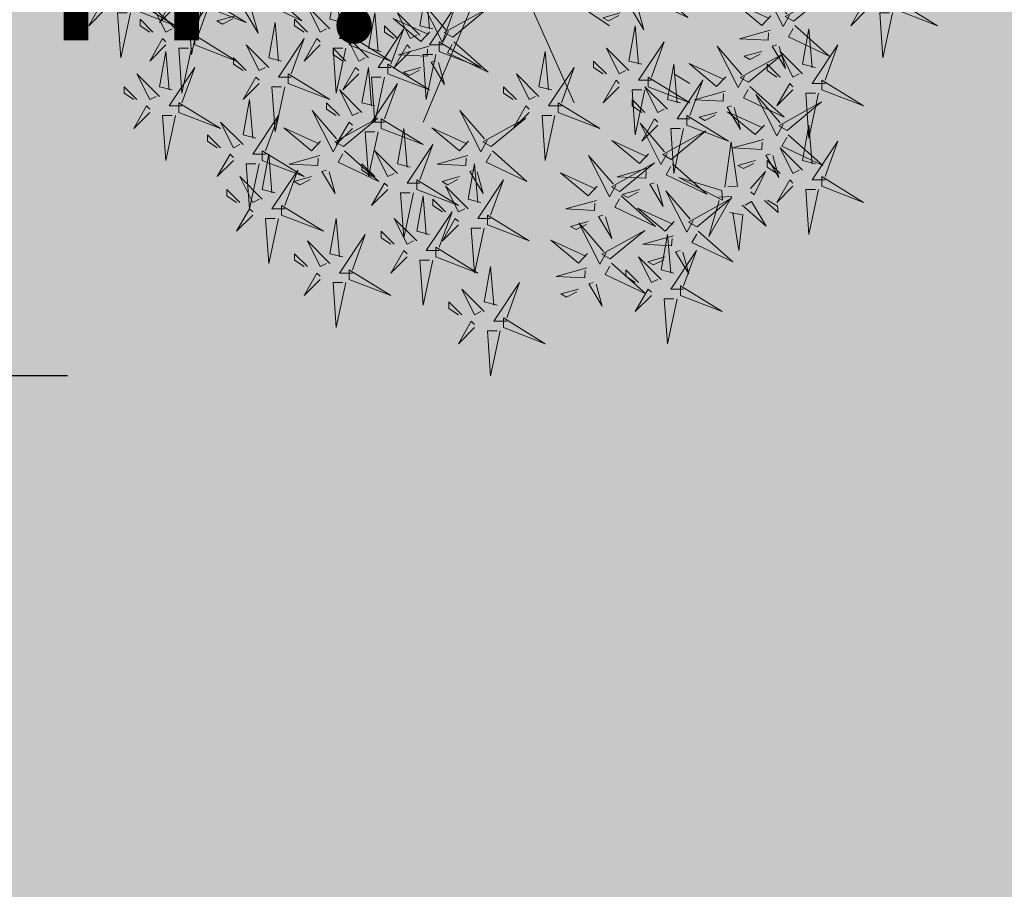
# Model space of a CAD drawing. Units: inches. Extents: x 1704 to 6393, y -157 to 1172.
# Tile 76 of 122: x 2017 to 2048, y 983 to 1009. Entities that reach past the tile are written whole.
import ezdxf

# ---------------------------------------------------------------- set-up
doc = ezdxf.new("R2010")
doc.units = ezdxf.units.IN
doc.header["$MEASUREMENT"] = 0
doc.layers.add('A-ANNO-DIMS', color=7, linetype='Continuous', lineweight=13)
doc.layers.add('L-shrub', color=74, linetype='Continuous', lineweight=18)
doc.layers.add('L-HRDS-PATT', color=9, linetype='Continuous', lineweight=13, true_color=0xc5c1ba)
doc.styles.get("Standard").update_dxf_attribs({"font": 'arial.ttf'})
doc.dimstyles.get("Standard").update_dxf_attribs({"dimtxt": 6, "dimasz": 2, "dimexe": 0.18, "dimexo": 0.0625, "dimgap": 0.09, "dimtad": 0, "dimtih": 1, "dimtoh": 1, "dimdec": 1, "dimzin": 0, "dimdsep": 46, "dimlunit": 3, "dimtxsty": 'Standard', "dimblk": 'ARCHTICK', "dimcen": 0.09, "dimadec": 0, "dimazin": 0, "dimtfac": 1, "dimtdec": 1, "dimtofl": 0, "dimtmove": 0, "dimatfit": 3, "dimfxl": 1, "dimtolj": 1, "dimtzin": 0, "dimarcsym": 0})

# ---------------------------------------------------------------- blocks, each defined once
blk = doc.blocks.new('autumn shrub')
at = {"layer": 'L-shrub'}
for p, q in [((11.54, 1.92), (51.94, 98)), ((1.92, -3.84), (-38.48, 86.47)), ((-98.12, 69.17), (-107.74, 74.94)), ((0, 0), (-59.64, 40.35)), ((71.18, 17.29), (98.12, 26.9)), ((9.62, -3.84), (71.18, 17.29)), ((11.54, -5.76), (55.79, 0)), ((-5.77, -9.61), (-38.48, -19.21)), ((1.92, -13.45), (-15.39, -86.47)), ((17.31, -26.9), (25.01, -40.35)), ((-76.95, -34.59), (-126.97, -48.04)), ((-67.33, -57.64), (-80.8, -63.41)), ((46.17, -69.17), (63.49, -101.84)), ((-17.31, -122.97), (-23.09, -155.64))]:
    blk.add_line(p, q, dxfattribs=at)
for points in [[(5.77, 222.89), (11.54, 249.79), (13.47, 222.89), (7.7, 222.89)], [(-100.04, 203.68), (-94.27, 230.58), (-92.34, 203.68), (-98.12, 203.68)], [(3.85, 220.97), (-21.16, 230.58), (3.85, 215.21), (3.85, 220.97)], [(21.16, 220.97), (30.78, 230.58), (23.09, 217.13), (21.16, 219.05)], [(98.12, 194.07), (103.89, 220.97), (105.81, 194.07), (100.04, 194.07)], [(1.92, 217.13), (9.62, 217.13), (-5.77, 194.07), (1.92, 215.21)], [(15.39, 211.36), (28.86, 197.91), (21.16, 213.28), (17.31, 211.36)], [(28.86, 213.28), (36.55, 205.6), (36.55, 209.44), (30.78, 213.28)], [(-101.96, 201.75), (-126.97, 211.36), (-101.96, 195.99), (-101.96, 201.75)], [(-84.65, 201.75), (-75.03, 211.36), (-82.73, 197.91), (-84.65, 199.83)], [(-51.51, 194.97), (-55.15, 208.07), (-47.22, 194.76), (-49.84, 194.03)], [(7.7, 207.52), (15.39, 205.6), (11.54, 184.46), (9.62, 207.52)], [(46.17, 180.62), (51.94, 207.52), (53.87, 180.62), (48.1, 180.62)], [(-60.75, 182.51), (-81.34, 200.76), (-56.96, 189.22), (-59.8, 184.19)], [(-41.04, 197.9), (-30.56, 200.83), (-33.91, 202.71), (-40.09, 199.58)], [(96.19, 192.15), (71.18, 201.75), (96.19, 186.38), (96.19, 192.15)], [(113.51, 192.15), (123.13, 201.75), (115.43, 188.3), (113.51, 190.23)], [(-103.89, 197.91), (-96.19, 197.91), (-111.58, 174.85), (-103.89, 195.99)], [(-103.45, 175.76), (-107.1, 188.86), (-99.16, 175.55), (-101.78, 174.81)], [(-90.42, 192.15), (-76.95, 178.7), (-84.65, 194.07), (-88.5, 192.15)], [(-76.95, 194.07), (-69.26, 186.38), (-69.26, 190.23), (-75.03, 194.07)], [(-45.98, 185.23), (-27.65, 190.35), (-44.82, 191.2), (-45.03, 186.9)], [(-98.12, 188.3), (-90.42, 186.38), (-94.27, 165.25), (-96.19, 188.3)], [(-92.98, 178.69), (-82.5, 181.61), (-85.85, 183.5), (-92.03, 180.36)], [(-57.62, 176.33), (-53.83, 183.03), (-41.31, 158.3), (-55.94, 175.38)], [(15.39, 161.4), (21.16, 188.3), (23.09, 161.4), (17.31, 161.4)], [(44.25, 178.7), (19.24, 188.3), (44.25, 172.93), (44.25, 178.7)], [(61.56, 178.7), (71.18, 188.3), (63.49, 174.85), (61.56, 176.78)], [(94.27, 188.3), (101.96, 188.3), (86.57, 165.25), (94.27, 186.38)], [(107.74, 182.54), (121.2, 169.09), (113.51, 184.46), (109.66, 182.54)], [(121.2, 184.46), (128.9, 176.78), (128.9, 180.62), (123.13, 184.46)], [(-112.69, 163.3), (-133.28, 181.54), (-108.91, 170), (-111.74, 164.97)], [(-60.02, 179.89), (-80.67, 162.83), (-55, 177.06), (-60.02, 179.89)], [(-46.41, 176.64), (-40.96, 182.39), (-24.44, 168.66), (-45.47, 178.31)], [(100.04, 178.7), (107.74, 176.78), (103.89, 155.64), (101.96, 178.7)], [(138.52, 155.64), (144.29, 182.54), (146.21, 155.64), (140.44, 155.64)], [(-131.51, 152.18), (-139.33, 153.55), (-136.98, 174.91), (-133.43, 152.04)], [(-97.92, 166.01), (-79.59, 171.13), (-96.76, 171.98), (-96.98, 167.69)], [(42.32, 174.85), (50.02, 174.85), (34.63, 151.8), (42.32, 172.93)], [(55.79, 169.09), (69.26, 155.64), (61.56, 171.01), (57.72, 169.09)], [(69.26, 171.01), (76.95, 163.33), (76.95, 167.17), (71.18, 171.01)], [(-184.69, 138.35), (-178.92, 165.25), (-176.99, 138.35), (-182.77, 138.35)], [(-125.08, 143), (-132.76, 142.46), (-119.03, 166.55), (-125.21, 144.92)], [(-57.28, 154.62), (-60.92, 167.72), (-52.99, 154.41), (-55.61, 153.68)], [(13.47, 159.48), (-11.54, 169.09), (13.47, 153.72), (13.47, 159.48)], [(30.78, 159.48), (40.4, 169.09), (32.71, 155.64), (30.78, 157.56)], [(48.1, 165.25), (55.79, 163.33), (51.94, 142.19), (50.02, 165.25)], [(57.72, 140.27), (63.49, 167.17), (65.41, 140.27), (59.64, 140.27)], [(-138.92, 147.8), (-153.3, 160.27), (-144.54, 145.48), (-140.84, 147.67)], [(-111.96, 160.68), (-132.62, 143.61), (-106.94, 157.85), (-111.96, 160.68)], [(-109.56, 157.11), (-105.78, 163.82), (-93.26, 139.08), (-107.89, 156.17)], [(-98.36, 157.42), (-92.9, 163.18), (-76.38, 149.44), (-97.41, 159.1)], [(-66.52, 142.16), (-87.11, 160.4), (-62.74, 148.86), (-65.57, 143.84)], [(-46.81, 157.55), (-36.33, 160.48), (-39.68, 162.36), (-45.86, 159.22)], [(136.59, 153.72), (111.58, 163.33), (136.59, 147.95), (136.59, 153.72)], [(153.91, 153.72), (163.53, 163.33), (155.83, 149.87), (153.91, 151.8)], [(11.54, 155.64), (19.24, 155.64), (3.85, 132.58), (11.54, 153.72)], [(-152.22, 144.94), (-160.44, 152.06), (-160.16, 148.23), (-154.14, 144.8)], [(-88.06, 135.41), (-91.71, 148.51), (-83.77, 135.2), (-86.39, 134.46)], [(-51.75, 144.88), (-33.42, 150), (-50.59, 150.85), (-50.8, 146.55)], [(25.01, 149.87), (38.48, 136.42), (30.78, 151.8), (26.93, 149.87)], [(55.79, 138.35), (30.78, 147.95), (55.79, 132.58), (55.79, 138.35)], [(38.48, 151.8), (46.17, 144.11), (46.17, 147.95), (40.4, 151.8)], [(73.11, 138.35), (82.73, 147.95), (75.03, 134.5), (73.11, 136.42)], [(134.67, 149.87), (142.36, 149.87), (126.97, 126.82), (134.67, 147.95)], [(150.06, 122.97), (155.83, 149.87), (157.76, 122.97), (151.98, 122.97)], [(-186.61, 136.42), (-211.62, 146.03), (-186.61, 130.66), (-186.61, 136.42)], [(-169.3, 136.42), (-159.68, 146.03), (-167.38, 132.58), (-169.3, 134.5)], [(-144, 137.81), (-152.92, 127.55), (-146.19, 141.51), (-144.13, 139.73)], [(-126.73, 139.03), (-101.1, 131.22), (-127.13, 144.78), (-126.73, 139.03)], [(-77.59, 138.33), (-67.11, 141.26), (-70.46, 143.15), (-76.64, 140.01)], [(-63.39, 135.98), (-59.61, 142.68), (-47.08, 117.95), (-61.71, 135.03)], [(-52.18, 136.28), (-46.73, 142.04), (-30.21, 128.31), (-51.24, 137.96)], [(17.31, 146.03), (25.01, 144.11), (21.16, 122.97), (19.24, 146.03)], [(148.14, 144.11), (161.6, 130.66), (153.91, 146.03), (150.06, 144.11)], [(161.6, 146.03), (169.3, 138.35), (169.3, 142.19), (163.53, 146.03)], [(-128.51, 136.98), (-132.37, 109.74), (-136.19, 136.44), (-130.43, 136.85)], [(-97.3, 122.95), (-117.89, 141.19), (-93.52, 129.65), (-96.35, 124.62)], [(-65.79, 139.54), (-86.44, 122.48), (-60.77, 136.71), (-65.79, 139.54)], [(19.67, 127.72), (16.03, 140.82), (23.96, 127.51), (21.35, 126.78)], [(108.17, 127.72), (104.53, 140.82), (112.46, 127.51), (109.84, 126.78)], [(140.44, 140.27), (148.14, 138.35), (144.29, 117.21), (142.36, 140.27)], [(-188.54, 132.58), (-180.84, 132.58), (-196.23, 109.52), (-188.54, 130.66)], [(-157.32, 118.11), (-160.96, 131.21), (-153.03, 117.9), (-155.65, 117.17)], [(-82.53, 125.66), (-64.2, 130.78), (-81.37, 131.63), (-81.59, 127.34)], [(10.44, 115.26), (-10.16, 133.5), (14.22, 121.96), (11.38, 116.94)], [(30.15, 130.65), (40.62, 133.58), (37.28, 135.46), (31.09, 132.32)], [(53.87, 134.5), (61.56, 134.5), (46.17, 111.45), (53.87, 132.58)], [(67.33, 128.74), (80.8, 115.29), (73.11, 130.66), (69.26, 128.74)], [(98.93, 115.26), (78.34, 133.5), (102.71, 121.96), (99.88, 116.94)], [(78.88, 103.76), (84.65, 130.66), (86.57, 103.76), (80.8, 103.76)], [(80.8, 130.66), (88.5, 122.97), (88.5, 126.82), (82.73, 130.66)], [(118.64, 130.65), (129.12, 133.58), (125.77, 135.46), (119.59, 132.32)], [(148.14, 121.05), (123.13, 130.66), (148.14, 115.29), (148.14, 121.05)], [(165.45, 121.05), (175.07, 130.66), (167.38, 117.21), (165.45, 119.13)], [(-166.56, 105.65), (-187.15, 123.9), (-162.78, 112.36), (-165.61, 107.33)], [(-175.07, 126.82), (-161.6, 113.37), (-169.3, 128.74), (-173.15, 126.82)], [(-161.6, 128.74), (-153.91, 121.05), (-153.91, 124.9), (-159.68, 128.74)], [(-146.85, 121.04), (-136.37, 123.97), (-139.72, 125.86), (-145.9, 122.72)], [(-103.89, 101.84), (-98.12, 128.74), (-96.19, 101.84), (-101.96, 101.84)], [(25.2, 117.98), (43.54, 123.1), (26.37, 123.95), (26.15, 119.65)], [(59.64, 124.9), (67.33, 122.97), (63.49, 101.84), (61.56, 124.9)], [(113.7, 117.98), (132.03, 123.1), (114.86, 123.95), (114.65, 119.65)], [(-182.77, 122.97), (-175.07, 121.05), (-178.92, 99.92), (-180.84, 122.97)], [(-96.57, 120.33), (-117.23, 103.26), (-91.55, 117.49), (-96.57, 120.33)], [(-94.17, 116.76), (-90.39, 123.47), (-77.87, 98.73), (-92.49, 115.82)], [(-82.96, 117.07), (-77.51, 122.83), (-60.99, 109.09), (-82.02, 118.75)], [(-26.93, 94.15), (-21.16, 121.05), (-19.24, 94.15), (-25.01, 94.15)], [(200.08, 94.15), (205.85, 121.05), (207.78, 94.15), (202, 94.15)], [(-151.79, 108.37), (-133.46, 113.49), (-150.63, 114.34), (-150.84, 110.04)], [(11.17, 112.64), (-9.49, 95.58), (16.19, 109.81), (11.17, 112.64)], [(13.57, 109.08), (17.35, 115.78), (29.87, 91.05), (15.24, 108.13)], [(24.77, 109.38), (30.23, 115.14), (46.74, 101.41), (25.72, 111.06)], [(99.66, 112.64), (79.01, 95.58), (104.68, 109.81), (99.66, 112.64)], [(102.06, 109.08), (105.85, 115.78), (118.37, 91.05), (103.74, 108.13)], [(113.27, 109.38), (118.72, 115.14), (135.24, 101.41), (114.21, 111.06)], [(146.21, 117.21), (153.91, 117.21), (138.52, 94.15), (146.21, 115.29)], [(159.68, 111.45), (173.15, 98), (165.45, 113.37), (161.6, 111.45)], [(173.15, 113.37), (180.84, 105.68), (180.84, 109.52), (175.07, 113.37)], [(-184.69, 80.7), (-178.92, 107.6), (-176.99, 80.7), (-182.77, 80.7)], [(-163.43, 99.47), (-159.65, 106.17), (-147.12, 81.44), (-161.75, 98.53)], [(-105.81, 99.92), (-130.82, 109.52), (-105.81, 94.15), (-105.81, 99.92)], [(-88.5, 99.92), (-78.88, 109.52), (-86.57, 96.07), (-88.5, 98)], [(76.95, 101.84), (51.94, 111.45), (76.95, 96.07), (76.95, 101.84)], [(94.27, 101.84), (103.89, 111.45), (96.19, 98), (94.27, 99.92)], [(151.98, 107.6), (159.68, 105.68), (155.83, 84.54), (153.91, 107.6)], [(-165.83, 103.03), (-186.48, 85.97), (-160.81, 100.2), (-165.83, 103.03)], [(-152.22, 99.78), (-146.77, 105.54), (-130.25, 91.8), (-151.28, 101.45)], [(-134.24, 89.29), (-137.88, 102.39), (-129.94, 89.08), (-132.56, 88.35)], [(-80.8, 78.78), (-75.03, 105.68), (-73.11, 78.78), (-78.88, 78.78)], [(-28.86, 92.23), (-53.87, 101.84), (-28.86, 86.47), (-28.86, 92.23)], [(-11.54, 92.23), (-1.92, 101.84), (-9.62, 88.39), (-11.54, 90.31)], [(134.67, 76.86), (140.44, 103.76), (142.36, 76.86), (136.59, 76.86)], [(198.16, 92.23), (173.15, 101.84), (198.16, 86.47), (198.16, 92.23)], [(215.47, 92.23), (225.09, 101.84), (217.4, 88.39), (215.47, 90.31)], [(-143.47, 76.83), (-164.07, 95.07), (-139.69, 83.53), (-142.53, 78.51)], [(-123.76, 92.22), (-113.29, 95.15), (-116.63, 97.03), (-122.82, 93.89)], [(-107.74, 96.07), (-100.04, 96.07), (-115.43, 73.02), (-107.74, 94.15)], [(75.03, 98), (82.73, 98), (67.33, 74.94), (75.03, 96.07)], [(75.03, 71.09), (80.8, 98), (82.73, 71.09), (76.95, 71.09)], [(-186.61, 78.78), (-211.62, 88.39), (-186.61, 73.02), (-186.61, 78.78)], [(-169.3, 78.78), (-159.68, 88.39), (-167.38, 74.94), (-169.3, 76.86)], [(-94.27, 90.31), (-80.8, 76.86), (-88.5, 92.23), (-92.34, 90.31)], [(-80.8, 92.23), (-73.11, 84.54), (-73.11, 88.39), (-78.88, 92.23)], [(-30.78, 88.39), (-23.09, 88.39), (-38.48, 65.33), (-30.78, 86.47)], [(80.8, 88.39), (88.5, 86.47), (84.65, 65.33), (82.73, 88.39)], [(88.5, 92.23), (101.96, 78.78), (94.27, 94.15), (90.42, 92.23)], [(101.96, 94.15), (109.66, 86.47), (109.66, 90.31), (103.89, 94.15)], [(196.23, 88.39), (203.93, 88.39), (188.54, 65.33), (196.23, 86.47)], [(-128.7, 79.55), (-110.37, 84.67), (-127.54, 85.52), (-127.76, 81.22)], [(-82.73, 76.86), (-107.74, 86.47), (-82.73, 71.09), (-82.73, 76.86)], [(-101.96, 86.47), (-94.27, 84.54), (-98.12, 63.41), (-100.04, 86.47)], [(-65.41, 76.86), (-55.79, 86.47), (-63.49, 73.02), (-65.41, 74.94)], [(-17.31, 82.62), (-3.85, 69.17), (-11.54, 84.54), (-15.39, 82.62)], [(-3.85, 84.54), (3.85, 76.86), (3.85, 80.7), (-1.92, 84.54)], [(44.25, 57.64), (50.02, 84.54), (51.94, 57.64), (46.17, 57.64)], [(132.75, 74.94), (107.74, 84.54), (132.75, 69.17), (132.75, 74.94)], [(150.06, 74.94), (159.68, 84.54), (151.98, 71.09), (150.06, 73.02)], [(209.7, 82.62), (223.17, 69.17), (215.47, 84.54), (211.62, 82.62)], [(223.17, 84.54), (230.86, 76.86), (230.86, 80.7), (225.09, 84.54)], [(-140.34, 70.65), (-136.56, 77.35), (-124.04, 52.62), (-138.67, 69.7)], [(-129.14, 70.95), (-123.68, 76.71), (-107.16, 62.98), (-128.19, 72.63)], [(-25.01, 78.78), (-17.31, 76.86), (-21.16, 55.72), (-23.09, 78.78)], [(73.11, 69.17), (48.1, 78.78), (73.11, 63.41), (73.11, 69.17)], [(90.42, 69.17), (100.04, 78.78), (92.34, 65.33), (90.42, 67.25)], [(98.12, 53.8), (103.89, 80.7), (105.81, 53.8), (100.04, 53.8)], [(190.46, 53.8), (196.23, 80.7), (198.16, 53.8), (192.39, 53.8)], [(202, 78.78), (209.7, 76.86), (205.85, 55.72), (203.93, 78.78)], [(-188.54, 74.94), (-180.84, 74.94), (-196.23, 51.88), (-188.54, 73.02)], [(-175.07, 69.17), (-161.6, 55.72), (-169.3, 71.09), (-173.15, 69.17)], [(-142.74, 74.21), (-163.4, 57.15), (-137.72, 71.38), (-142.74, 74.21)], [(-161.6, 71.09), (-153.91, 63.41), (-153.91, 67.25), (-159.68, 71.09)], [(-84.65, 73.02), (-76.95, 73.02), (-92.34, 49.96), (-84.65, 71.09)], [(42.76, 62.39), (39.12, 75.49), (47.05, 62.18), (44.43, 61.45)], [(130.82, 71.09), (138.52, 71.09), (123.13, 48.04), (130.82, 69.17)], [(-182.77, 65.33), (-175.07, 63.41), (-178.92, 42.27), (-180.84, 65.33)], [(-161.17, 52.78), (-164.81, 65.88), (-156.88, 52.57), (-159.5, 51.84)], [(-71.18, 67.25), (-57.72, 53.8), (-65.41, 69.17), (-69.26, 67.25)], [(-57.72, 69.17), (-50.02, 61.49), (-50.02, 65.33), (-55.79, 69.17)], [(33.52, 49.93), (12.93, 68.17), (37.3, 56.63), (34.47, 51.61)], [(42.32, 55.72), (17.31, 65.33), (42.32, 49.96), (42.32, 55.72)], [(53.23, 65.32), (63.71, 68.25), (60.36, 70.13), (54.18, 66.99)], [(59.64, 55.72), (69.26, 65.33), (61.56, 51.88), (59.64, 53.8)], [(71.18, 65.33), (78.88, 65.33), (63.49, 42.27), (71.18, 63.41)], [(144.29, 65.33), (157.76, 51.88), (150.06, 67.25), (146.21, 65.33)], [(157.76, 67.25), (165.45, 59.57), (165.45, 63.41), (159.68, 67.25)], [(-228.94, 32.67), (-223.17, 59.57), (-221.24, 32.67), (-227.01, 32.67)], [(-150.69, 55.71), (-140.22, 58.64), (-143.57, 60.53), (-149.75, 57.39)], [(-78.88, 63.41), (-71.18, 61.49), (-75.03, 40.35), (-76.95, 63.41)], [(96.19, 51.88), (71.18, 61.49), (96.19, 46.12), (96.19, 51.88)], [(84.65, 59.57), (98.12, 46.12), (90.42, 61.49), (86.57, 59.57)], [(98.12, 61.49), (105.81, 53.8), (105.81, 57.64), (100.04, 61.49)], [(113.51, 51.88), (123.13, 61.49), (115.43, 48.04), (113.51, 49.96)], [(136.59, 61.49), (144.29, 59.57), (140.44, 38.43), (138.52, 61.49)], [(188.54, 51.88), (163.53, 61.49), (188.54, 46.12), (188.54, 51.88)], [(205.85, 51.88), (215.47, 61.49), (207.78, 48.04), (205.85, 49.96)], [(227.01, 32.67), (232.79, 59.57), (234.71, 32.67), (228.94, 32.67)], [(-170.4, 40.32), (-191, 58.57), (-166.62, 47.03), (-169.46, 42)], [(48.29, 52.64), (66.62, 57.77), (49.45, 58.62), (49.24, 54.32)], [(76.95, 55.72), (84.65, 53.8), (80.8, 32.67), (78.88, 55.72)], [(184.69, 30.74), (190.46, 57.64), (192.39, 30.74), (186.61, 30.74)], [(-155.64, 43.04), (-137.31, 48.16), (-154.48, 49.01), (-154.69, 44.71)], [(34.25, 47.31), (13.6, 30.25), (39.27, 44.48), (34.25, 47.31)], [(40.4, 51.88), (48.1, 51.88), (32.71, 28.82), (40.4, 49.96)], [(36.65, 43.75), (40.43, 50.45), (52.96, 25.72), (38.33, 42.8)], [(47.86, 44.05), (53.31, 49.81), (69.83, 36.08), (48.8, 45.73)], [(53.87, 46.12), (67.33, 32.67), (59.64, 48.04), (55.79, 46.12)], [(67.33, 48.04), (75.03, 40.35), (75.03, 44.19), (69.26, 48.04)], [(94.27, 48.04), (101.96, 48.04), (86.57, 24.98), (94.27, 46.12)], [(186.61, 48.04), (194.31, 48.04), (178.92, 24.98), (186.61, 46.12)], [(-76.52, 29.73), (-80.16, 42.83), (-72.23, 29.51), (-74.85, 28.78)], [(46.17, 42.27), (53.87, 40.35), (50.02, 19.21), (48.1, 42.27)], [(107.74, 42.27), (121.2, 28.82), (113.51, 44.19), (109.66, 42.27)], [(121.2, 44.19), (128.9, 36.51), (128.9, 40.35), (123.13, 44.19)], [(154.34, 31.65), (150.7, 44.75), (158.63, 31.44), (156.02, 30.7)], [(200.08, 42.27), (213.55, 28.82), (205.85, 44.19), (202, 42.27)], [(213.55, 44.19), (221.24, 36.51), (221.24, 40.35), (215.47, 44.19)], [(-230.86, 30.74), (-255.87, 40.35), (-230.86, 24.98), (-230.86, 30.74)], [(-213.55, 30.74), (-203.93, 40.35), (-211.62, 26.9), (-213.55, 28.82)], [(-169.68, 37.7), (-190.33, 20.64), (-164.66, 34.87), (-169.68, 37.7)], [(-167.27, 34.14), (-163.49, 40.84), (-150.97, 16.11), (-165.6, 33.2)], [(-156.07, 34.45), (-150.62, 40.21), (-134.1, 26.47), (-155.13, 36.12)], [(-85.76, 17.27), (-106.35, 35.51), (-81.97, 23.97), (-84.81, 18.94)], [(-66.05, 32.65), (-55.57, 35.58), (-58.92, 37.47), (-65.1, 34.33)], [(100.04, 38.43), (107.74, 36.51), (103.89, 15.37), (101.96, 38.43)], [(145.11, 19.19), (124.51, 37.43), (148.89, 25.89), (146.05, 20.86)], [(182.77, 28.82), (157.76, 38.43), (182.77, 23.06), (182.77, 28.82)], [(164.82, 34.57), (175.29, 37.5), (171.94, 39.39), (165.76, 36.25)], [(192.39, 38.43), (200.08, 36.51), (196.23, 15.37), (194.31, 38.43)], [(225.09, 30.74), (200.08, 40.35), (225.09, 24.98), (225.09, 30.74)], [(200.08, 28.82), (209.7, 38.43), (202, 24.98), (200.08, 26.9)], [(242.41, 30.74), (252.02, 40.35), (244.33, 26.9), (242.41, 28.82)], [(-232.79, 26.9), (-225.09, 26.9), (-240.48, 3.84), (-232.79, 24.98)], [(-70.99, 19.98), (-52.66, 25.1), (-69.83, 25.95), (-70.04, 21.66)], [(159.87, 21.9), (178.21, 27.02), (161.04, 27.87), (160.82, 23.58)], [(180.84, 24.98), (188.54, 24.98), (173.15, 1.92), (180.84, 23.06)], [(223.17, 26.9), (230.86, 26.9), (215.47, 3.84), (223.17, 24.98)], [(215.47, -1.92), (221.24, 24.98), (223.17, -1.92), (217.4, -1.92)], [(-219.32, 21.14), (-205.85, 7.69), (-213.55, 23.06), (-217.4, 21.14)], [(-213.55, -3.84), (-207.78, 23.06), (-205.85, -3.84), (-211.62, -3.84)], [(-205.85, 23.06), (-198.16, 15.37), (-198.16, 19.21), (-203.93, 23.06)], [(-161.6, -7.69), (-155.83, 19.21), (-153.91, -7.69), (-159.68, -7.69)], [(-96.19, -5.76), (-90.42, 21.14), (-88.5, -5.76), (-94.27, -5.76)], [(-82.63, 11.08), (-78.84, 17.78), (-66.32, -6.95), (-80.95, 10.14)], [(-57.72, -3.84), (-51.94, 23.06), (-50.02, -3.84), (-55.79, -3.84)], [(148.24, 13), (152.02, 19.71), (164.54, -5.03), (149.91, 12.06)], [(159.44, 13.31), (164.89, 19.07), (181.41, 5.33), (160.39, 14.99)], [(194.31, 19.21), (207.78, 5.76), (200.08, 21.14), (196.23, 19.21)], [(207.78, 21.14), (215.47, 13.45), (215.47, 17.29), (209.7, 21.14)], [(236.63, 21.14), (250.1, 7.69), (242.41, 23.06), (238.56, 21.14)], [(250.1, 23.06), (257.8, 15.37), (257.8, 19.21), (252.02, 23.06)], [(-227.01, 17.29), (-219.32, 15.37), (-223.17, -5.76), (-225.09, 17.29)], [(-85.03, 14.65), (-105.68, -2.42), (-80.01, 11.81), (-85.03, 14.65)], [(-71.42, 11.39), (-65.97, 17.15), (-49.45, 3.41), (-70.48, 13.06)], [(34.63, -9.61), (40.4, 17.29), (42.32, -9.61), (36.55, -9.61)], [(145.83, 16.57), (125.18, -0.5), (150.86, 13.74), (145.83, 16.57)], [(186.61, 15.37), (194.31, 13.45), (190.46, -7.69), (188.54, 15.37)], [(228.94, 17.29), (236.63, 15.37), (232.79, -5.76), (230.86, 17.29)], [(-215.47, -5.76), (-240.48, 3.84), (-215.47, -11.53), (-215.47, -5.76)], [(-198.16, -5.76), (-188.54, 3.84), (-196.23, -9.61), (-198.16, -7.69)], [(-163.53, -9.61), (-188.54, 0), (-163.53, -15.37), (-163.53, -9.61)], [(-146.21, -9.61), (-136.59, 0), (-144.29, -13.45), (-146.21, -11.53)], [(-98.12, -7.69), (-123.13, 1.92), (-98.12, -13.45), (-98.12, -7.69)], [(-59.64, -5.76), (-84.65, 3.84), (-59.64, -11.53), (-59.64, -5.76)], [(-80.8, -7.69), (-71.18, 1.92), (-78.88, -11.53), (-80.8, -9.61)], [(-42.32, -5.76), (-32.71, 3.84), (-40.4, -9.61), (-42.32, -7.69)], [(110.09, -10.62), (106.45, 2.47), (114.39, -10.84), (111.77, -11.57)], [(213.55, -3.84), (188.54, 5.76), (213.55, -9.61), (213.55, -3.84)], [(230.86, -3.84), (240.48, 5.76), (232.79, -7.69), (230.86, -5.76)], [(232.79, -26.9), (238.56, 0), (240.48, -26.9), (234.71, -26.9)], [(32.71, -11.53), (7.7, -1.92), (32.71, -17.29), (32.71, -11.53)], [(50.02, -11.53), (59.64, -1.92), (51.94, -15.37), (50.02, -13.45)], [(100.86, -23.09), (80.26, -4.84), (104.64, -16.38), (101.8, -21.41)], [(120.57, -7.7), (131.04, -4.77), (127.7, -2.88), (121.51, -6.02)], [(-217.4, -9.61), (-209.7, -9.61), (-225.09, -32.67), (-217.4, -11.53)], [(-100.04, -11.53), (-92.34, -11.53), (-107.74, -34.59), (-100.04, -13.45)], [(-61.56, -9.61), (-53.87, -9.61), (-69.26, -32.67), (-61.56, -11.53)], [(211.62, -7.69), (219.32, -7.69), (203.93, -30.74), (211.62, -9.61)], [(225.09, -13.45), (238.56, -26.9), (230.86, -11.53), (227.01, -13.45)], [(238.56, -11.53), (246.25, -19.21), (246.25, -15.37), (240.48, -11.53)], [(-203.93, -15.37), (-190.46, -28.82), (-198.16, -13.45), (-202, -15.37)], [(-190.46, -13.45), (-182.77, -21.14), (-182.77, -17.29), (-188.54, -13.45)], [(-165.45, -13.45), (-157.76, -13.45), (-173.15, -36.51), (-165.45, -15.37)], [(-151.98, -19.21), (-138.52, -32.67), (-146.21, -17.29), (-150.06, -19.21)], [(-138.52, -17.29), (-130.82, -24.98), (-130.82, -21.14), (-136.59, -17.29)], [(-86.57, -17.29), (-73.11, -30.74), (-80.8, -15.37), (-84.65, -17.29)], [(-78.88, -44.19), (-73.11, -17.29), (-71.18, -44.19), (-76.95, -44.19)], [(-73.11, -15.37), (-65.41, -23.06), (-65.41, -19.21), (-71.18, -15.37)], [(-48.1, -15.37), (-34.63, -28.82), (-42.32, -13.45), (-46.17, -15.37)], [(-34.63, -13.45), (-26.93, -21.14), (-26.93, -17.29), (-32.71, -13.45)], [(30.78, -15.37), (38.48, -15.37), (23.09, -38.43), (30.78, -17.29)], [(115.63, -20.37), (133.96, -15.25), (116.79, -14.4), (116.57, -18.7)], [(217.4, -17.29), (225.09, -19.21), (221.24, -40.35), (219.32, -17.29)], [(-228.94, -48.04), (-223.17, -21.14), (-221.24, -48.04), (-227.01, -48.04)], [(-211.62, -19.21), (-203.93, -21.14), (-207.78, -42.27), (-209.7, -19.21)], [(-159.68, -23.06), (-151.98, -24.98), (-155.83, -46.12), (-157.76, -23.06)], [(-94.27, -21.14), (-86.57, -23.06), (-90.42, -44.19), (-92.34, -21.14)], [(-55.79, -19.21), (-48.1, -21.14), (-51.94, -42.27), (-53.87, -19.21)], [(44.25, -21.14), (57.72, -34.59), (50.02, -19.21), (46.17, -21.14)], [(57.72, -19.21), (65.41, -26.9), (65.41, -23.06), (59.64, -19.21)], [(103.99, -29.27), (107.77, -22.57), (120.29, -47.3), (105.66, -30.21)], [(115.19, -28.96), (120.65, -23.2), (137.17, -36.94), (116.14, -27.29)], [(230.86, -28.82), (205.85, -19.21), (230.86, -34.59), (230.86, -28.82)], [(248.18, -28.82), (257.8, -19.21), (250.1, -32.67), (248.18, -30.74)], [(36.55, -24.98), (44.25, -26.9), (40.4, -48.04), (38.48, -24.98)], [(71.18, -53.8), (76.95, -26.9), (78.88, -53.8), (73.11, -53.8)], [(101.59, -25.71), (80.93, -42.77), (106.61, -28.54), (101.59, -25.71)], [(173.15, -55.72), (178.92, -28.82), (180.84, -55.72), (175.07, -55.72)], [(40.4, -59.57), (46.17, -32.67), (48.1, -59.57), (42.32, -59.57)], [(111.58, -61.49), (117.35, -34.59), (119.28, -61.49), (113.51, -61.49)], [(228.94, -32.67), (236.63, -32.67), (221.24, -55.72), (228.94, -34.59)], [(-230.86, -49.96), (-255.87, -40.35), (-230.86, -55.72), (-230.86, -49.96)], [(-213.55, -49.96), (-203.93, -40.35), (-211.62, -53.8), (-213.55, -51.88)], [(-141.93, -52.9), (-145.57, -39.8), (-137.64, -53.11), (-140.26, -53.84)], [(-80.8, -46.12), (-105.81, -36.51), (-80.8, -51.88), (-80.8, -46.12)], [(-63.49, -46.12), (-53.87, -36.51), (-61.56, -49.96), (-63.49, -48.04)], [(242.41, -38.43), (255.87, -51.88), (248.18, -36.51), (244.33, -38.43)], [(255.87, -36.51), (263.57, -44.19), (263.57, -40.35), (257.8, -36.51)], [(-188.54, -69.17), (-182.77, -42.27), (-180.84, -69.17), (-186.61, -69.17)], [(-151.17, -65.36), (-171.76, -47.11), (-147.39, -58.66), (-150.22, -63.68)], [(-131.46, -49.97), (-120.98, -47.04), (-124.33, -45.16), (-130.51, -48.29)], [(69.26, -55.72), (44.25, -46.12), (69.26, -61.49), (69.26, -55.72)], [(86.57, -55.72), (96.19, -46.12), (88.5, -59.57), (86.57, -57.64)], [(234.71, -42.27), (242.41, -44.19), (238.56, -65.33), (236.63, -42.27)], [(-82.73, -49.96), (-75.03, -49.96), (-90.42, -73.02), (-82.73, -51.88)], [(-30.78, -76.86), (-25.01, -49.96), (-23.09, -76.86), (-28.86, -76.86)], [(38.48, -61.49), (13.47, -51.88), (38.48, -67.25), (38.48, -61.49)], [(55.79, -61.49), (65.41, -51.88), (57.72, -65.33), (55.79, -63.41)], [(171.22, -57.64), (146.21, -48.04), (171.22, -63.41), (171.22, -57.64)], [(188.54, -57.64), (198.16, -48.04), (190.46, -61.49), (188.54, -59.57)], [(-232.79, -53.8), (-225.09, -53.8), (-240.48, -76.86), (-232.79, -55.72)], [(-219.32, -59.57), (-205.85, -73.02), (-213.55, -57.64), (-217.4, -59.57)], [(-205.85, -57.64), (-198.16, -65.33), (-198.16, -61.49), (-203.93, -57.64)], [(-136.4, -62.64), (-118.07, -57.52), (-135.24, -56.67), (-135.45, -60.97)], [(-76.95, -80.7), (-71.18, -53.8), (-69.26, -80.7), (-75.03, -80.7)], [(-69.26, -55.72), (-55.79, -69.17), (-63.49, -53.8), (-67.33, -55.72)], [(-55.79, -53.8), (-48.1, -61.49), (-48.1, -57.64), (-53.87, -53.8)], [(71.18, -84.54), (76.95, -57.64), (78.88, -84.54), (73.11, -84.54)], [(109.66, -63.41), (84.65, -53.8), (109.66, -69.17), (109.66, -63.41)], [(126.97, -63.41), (136.59, -53.8), (128.9, -67.25), (126.97, -65.33)], [(211.62, -82.62), (217.4, -55.72), (219.32, -82.62), (213.55, -82.62)], [(-227.01, -63.41), (-219.32, -65.33), (-223.17, -86.47), (-225.09, -63.41)], [(-190.46, -71.09), (-215.47, -61.49), (-190.46, -76.86), (-190.46, -71.09)], [(-173.15, -71.09), (-163.53, -61.49), (-171.22, -74.94), (-173.15, -73.02)], [(-76.95, -59.57), (-69.26, -61.49), (-73.11, -82.62), (-75.03, -59.57)], [(67.33, -59.57), (75.03, -59.57), (59.64, -82.62), (67.33, -61.49)], [(80.8, -65.33), (94.27, -78.78), (86.57, -63.41), (82.73, -65.33)], [(94.27, -63.41), (101.96, -71.09), (101.96, -67.25), (96.19, -63.41)], [(169.3, -61.49), (176.99, -61.49), (161.6, -84.54), (169.3, -63.41)], [(-150.44, -67.98), (-171.09, -85.04), (-145.42, -70.81), (-150.44, -67.98)], [(-148.04, -71.54), (-144.26, -64.84), (-131.73, -89.57), (-146.36, -72.49)], [(-142.36, -96.07), (-136.59, -69.17), (-134.67, -96.07), (-140.44, -96.07)], [(-136.83, -71.23), (-131.38, -65.48), (-114.86, -79.21), (-135.89, -69.56)], [(-32.71, -78.78), (-57.72, -69.17), (-32.71, -84.54), (-32.71, -78.78)], [(-15.39, -78.78), (-5.77, -69.17), (-13.47, -82.62), (-15.39, -80.7)], [(36.55, -65.33), (44.25, -65.33), (28.86, -88.39), (36.55, -67.25)], [(50.02, -71.09), (63.49, -84.54), (55.79, -69.17), (51.94, -71.09)], [(63.49, -69.17), (71.18, -76.86), (71.18, -73.02), (65.41, -69.17)], [(73.11, -69.17), (80.8, -71.09), (76.95, -92.23), (75.03, -69.17)], [(107.74, -67.25), (115.43, -67.25), (100.04, -90.31), (107.74, -69.17)], [(150.49, -79.8), (146.85, -66.7), (154.79, -80.01), (152.17, -80.74)], [(182.77, -67.25), (196.23, -80.7), (188.54, -65.33), (184.69, -67.25)], [(196.23, -65.33), (203.93, -73.02), (203.93, -69.17), (198.16, -65.33)], [(-192.39, -74.94), (-184.69, -74.94), (-200.08, -98), (-192.39, -76.86)], [(-78.88, -82.62), (-103.89, -73.02), (-78.88, -88.39), (-78.88, -82.62)], [(-61.56, -82.62), (-51.94, -73.02), (-59.64, -86.47), (-61.56, -84.54)], [(42.32, -74.94), (50.02, -76.86), (46.17, -98), (44.25, -74.94)], [(141.26, -92.26), (120.66, -74.02), (145.04, -85.56), (142.2, -90.58)], [(121.2, -73.02), (134.67, -86.47), (126.97, -71.09), (123.13, -73.02)], [(134.67, -71.09), (142.36, -78.78), (142.36, -74.94), (136.59, -71.09)], [(160.97, -76.87), (171.44, -73.94), (168.1, -72.06), (161.91, -75.19)], [(175.07, -71.09), (182.77, -73.02), (178.92, -94.15), (176.99, -71.09)], [(209.7, -84.54), (184.69, -74.94), (209.7, -90.31), (209.7, -84.54)], [(227.01, -84.54), (236.63, -74.94), (228.94, -88.39), (227.01, -86.47)], [(-178.92, -80.7), (-165.45, -94.15), (-173.15, -78.78), (-176.99, -80.7)], [(-165.45, -78.78), (-157.76, -86.47), (-157.76, -82.62), (-163.53, -78.78)], [(69.26, -86.47), (44.25, -76.86), (69.26, -92.23), (69.26, -86.47)], [(86.57, -86.47), (96.19, -76.86), (88.5, -90.31), (86.57, -88.39)], [(113.51, -76.86), (121.2, -78.78), (117.35, -99.92), (115.43, -76.86)], [(-186.61, -84.54), (-178.92, -86.47), (-182.77, -107.6), (-184.69, -84.54)], [(-80.8, -86.47), (-73.11, -86.47), (-88.5, -109.52), (-80.8, -88.39)], [(-34.63, -82.62), (-26.93, -82.62), (-42.32, -105.68), (-34.63, -84.54)], [(-21.16, -88.39), (-7.7, -101.84), (-15.39, -86.47), (-19.24, -88.39)], [(-7.7, -86.47), (0, -94.15), (0, -90.31), (-5.77, -86.47)], [(156.03, -89.54), (174.36, -84.42), (157.19, -83.57), (156.97, -87.87)], [(-144.29, -98), (-169.3, -88.39), (-144.29, -103.76), (-144.29, -98)], [(-126.97, -98), (-117.35, -88.39), (-125.05, -101.84), (-126.97, -99.92)], [(-67.33, -92.23), (-53.87, -105.68), (-61.56, -90.31), (-65.41, -92.23)], [(-53.87, -90.31), (-46.17, -98), (-46.17, -94.15), (-51.94, -90.31)], [(-28.86, -92.23), (-21.16, -94.15), (-25.01, -115.29), (-26.93, -92.23)], [(67.33, -90.31), (75.03, -90.31), (59.64, -113.37), (67.33, -92.23)], [(80.8, -96.07), (94.27, -109.52), (86.57, -94.15), (82.73, -96.07)], [(94.27, -94.15), (101.96, -101.84), (101.96, -98), (96.19, -94.15)], [(144.39, -98.44), (148.17, -91.74), (160.69, -116.47), (146.06, -99.39)], [(155.59, -98.13), (161.05, -92.38), (177.57, -106.11), (156.54, -96.46)], [(186.61, -115.29), (192.39, -88.39), (194.31, -115.29), (188.54, -115.29)], [(207.78, -88.39), (215.47, -88.39), (200.08, -111.45), (207.78, -90.31)], [(221.24, -94.15), (234.71, -107.6), (227.01, -92.23), (223.17, -94.15)], [(234.71, -92.23), (242.41, -99.92), (242.41, -96.07), (236.63, -92.23)], [(-75.03, -96.07), (-67.33, -98), (-71.18, -119.13), (-73.11, -96.07)], [(73.11, -99.92), (80.8, -101.84), (76.95, -122.97), (75.03, -99.92)], [(141.99, -94.88), (121.33, -111.94), (147.01, -97.71), (141.99, -94.88)], [(213.55, -98), (221.24, -99.92), (217.4, -121.05), (215.47, -98)], [(-146.21, -101.84), (-138.52, -101.84), (-153.91, -124.9), (-146.21, -103.76)], [(-132.75, -107.6), (-119.28, -121.05), (-126.97, -105.68), (-130.82, -107.6)], [(-119.28, -105.68), (-111.58, -113.37), (-111.58, -109.52), (-117.35, -105.68)], [(-88.06, -118.23), (-91.71, -105.13), (-83.77, -118.44), (-86.39, -119.17)], [(10.05, -118.23), (6.41, -105.13), (14.35, -118.44), (11.73, -119.17)], [(78.88, -128.74), (84.65, -101.84), (86.57, -128.74), (80.8, -128.74)], [(-140.44, -111.45), (-132.75, -113.37), (-136.59, -134.5), (-138.52, -111.45)], [(-130.82, -134.5), (-125.05, -107.6), (-123.13, -134.5), (-128.9, -134.5)], [(-77.59, -115.3), (-67.11, -112.37), (-70.46, -110.49), (-76.64, -113.62)], [(20.53, -115.3), (31, -112.37), (27.66, -110.49), (21.47, -113.62)], [(184.69, -117.21), (159.68, -107.6), (184.69, -122.97), (184.69, -117.21)], [(202, -117.21), (211.62, -107.6), (203.93, -121.05), (202, -119.13)], [(-182.77, -142.19), (-176.99, -115.29), (-175.07, -142.19), (-180.84, -142.19)], [(-97.3, -130.69), (-117.89, -112.44), (-93.52, -123.99), (-96.35, -129.01)], [(0.82, -130.69), (-19.78, -112.44), (4.6, -123.99), (1.76, -129.01)], [(127.41, -125.91), (123.77, -112.81), (131.7, -126.12), (129.08, -126.86)], [(-82.53, -127.97), (-64.2, -122.85), (-81.37, -122), (-81.59, -126.3)], [(15.59, -127.97), (33.92, -122.85), (16.75, -122), (16.53, -126.3)], [(76.95, -130.66), (51.94, -121.05), (76.95, -136.42), (76.95, -130.66)], [(53.87, -146.03), (59.64, -119.13), (61.56, -146.03), (55.79, -146.03)], [(94.27, -130.66), (103.89, -121.05), (96.19, -134.5), (94.27, -132.58)], [(118.17, -138.37), (97.58, -120.13), (121.95, -131.67), (119.12, -136.7)], [(137.88, -122.99), (148.36, -120.06), (145.01, -118.17), (138.83, -121.31)], [(163.53, -146.03), (169.3, -119.13), (171.22, -146.03), (165.45, -146.03)], [(182.77, -121.05), (190.46, -121.05), (175.07, -144.11), (182.77, -122.97)], [(-132.75, -136.42), (-157.76, -126.82), (-132.75, -142.19), (-132.75, -136.42)], [(-115.43, -136.42), (-105.81, -126.82), (-113.51, -140.27), (-115.43, -138.35)], [(196.23, -126.82), (209.7, -140.27), (202, -124.9), (198.16, -126.82)], [(209.7, -124.9), (217.4, -132.58), (217.4, -128.74), (211.62, -124.9)], [(-184.69, -144.11), (-209.7, -134.5), (-184.69, -149.87), (-184.69, -144.11)], [(-167.38, -144.11), (-157.76, -134.5), (-165.45, -147.95), (-167.38, -146.03)], [(-96.57, -133.31), (-117.23, -150.37), (-91.55, -136.14), (-96.57, -133.31)], [(-94.17, -136.87), (-90.39, -130.17), (-77.87, -154.9), (-92.49, -137.82)], [(-82.96, -136.56), (-77.51, -130.81), (-60.99, -144.54), (-82.02, -134.89)], [(-82.73, -157.56), (-76.95, -130.66), (-75.03, -157.56), (-80.8, -157.56)], [(-39.97, -145.13), (-43.61, -132.03), (-35.67, -145.34), (-38.29, -146.07)], [(1.55, -133.31), (-19.11, -150.37), (6.57, -136.14), (1.55, -133.31)], [(3.95, -136.87), (7.73, -130.17), (20.25, -154.9), (5.62, -137.82)], [(15.15, -136.56), (20.61, -130.81), (37.13, -144.54), (16.1, -134.89)], [(75.03, -134.5), (82.73, -134.5), (67.33, -157.56), (75.03, -136.42)], [(132.94, -135.66), (151.27, -130.54), (134.1, -129.69), (133.89, -133.98)], [(188.54, -130.66), (196.23, -132.58), (192.39, -153.72), (190.46, -130.66)], [(-134.67, -140.27), (-126.97, -140.27), (-142.36, -163.33), (-134.67, -142.19)], [(-49.2, -157.59), (-69.8, -139.35), (-45.42, -150.89), (-48.26, -155.91)], [(-29.49, -142.2), (-19.02, -139.27), (-22.36, -137.39), (-28.55, -140.52)], [(51.94, -147.95), (26.93, -138.35), (51.94, -153.72), (51.94, -147.95)], [(69.26, -147.95), (78.88, -138.35), (71.18, -151.8), (69.26, -149.87)], [(88.5, -140.27), (101.96, -153.72), (94.27, -138.35), (90.42, -140.27)], [(118.9, -140.99), (98.25, -158.06), (123.92, -143.83), (118.9, -140.99)], [(101.96, -138.35), (109.66, -146.03), (109.66, -142.19), (103.89, -138.35)], [(121.3, -144.56), (125.08, -137.85), (137.61, -162.59), (122.98, -145.5)], [(132.51, -144.25), (137.96, -138.49), (154.48, -152.23), (133.45, -142.57)], [(161.6, -147.95), (136.59, -138.35), (161.6, -153.72), (161.6, -147.95)], [(178.92, -147.95), (188.54, -138.35), (180.84, -151.8), (178.92, -149.87)], [(-121.2, -146.03), (-107.74, -159.48), (-115.43, -144.11), (-119.28, -146.03)], [(-107.74, -144.11), (-100.04, -151.8), (-100.04, -147.95), (-105.81, -144.11)], [(80.8, -144.11), (88.5, -146.03), (84.65, -167.17), (82.73, -144.11)], [(-186.61, -147.95), (-178.92, -147.95), (-194.31, -171.01), (-186.61, -149.87)], [(-173.15, -153.72), (-159.68, -167.17), (-167.38, -151.8), (-171.22, -153.72)], [(-159.68, -151.8), (-151.98, -159.48), (-151.98, -155.64), (-157.76, -151.8)], [(-128.9, -149.87), (-121.2, -151.8), (-125.05, -172.93), (-126.97, -149.87)], [(-84.65, -159.48), (-109.66, -149.87), (-84.65, -165.25), (-84.65, -159.48)], [(-67.33, -159.48), (-57.72, -149.87), (-65.41, -163.33), (-67.33, -161.4)], [(-36.55, -176.78), (-30.78, -149.87), (-28.86, -176.78), (-34.63, -176.78)], [(-34.43, -154.87), (-16.1, -149.75), (-33.27, -148.9), (-33.49, -153.2)], [(50.02, -151.8), (57.72, -151.8), (42.32, -174.85), (50.02, -153.72)], [(159.68, -151.8), (167.38, -151.8), (151.98, -174.85), (159.68, -153.72)], [(-180.84, -157.56), (-173.15, -159.48), (-176.99, -180.62), (-178.92, -157.56)], [(-46.07, -163.77), (-42.29, -157.07), (-29.77, -181.8), (-44.4, -164.72)], [(-34.87, -163.46), (-29.41, -157.71), (-12.89, -171.44), (-33.92, -161.79)], [(9.62, -184.46), (15.39, -157.56), (17.31, -184.46), (11.54, -184.46)], [(63.49, -157.56), (76.95, -171.01), (69.26, -155.64), (65.41, -157.56)], [(76.95, -155.64), (84.65, -163.33), (84.65, -159.48), (78.88, -155.64)], [(112.02, -172.03), (108.37, -158.93), (116.31, -172.24), (113.69, -172.97)], [(173.15, -157.56), (186.61, -171.01), (178.92, -155.64), (175.07, -157.56)], [(186.61, -155.64), (194.31, -163.33), (194.31, -159.48), (188.54, -155.64)], [(-103.89, -190.23), (-98.12, -163.33), (-96.19, -190.23), (-101.96, -190.23)], [(-86.57, -163.33), (-78.88, -163.33), (-94.27, -186.38), (-86.57, -165.25)], [(-48.47, -160.21), (-69.13, -177.27), (-43.45, -163.04), (-48.47, -160.21)], [(42.76, -175.87), (39.12, -162.77), (47.05, -176.08), (44.43, -176.81)], [(55.79, -161.4), (63.49, -163.33), (59.64, -184.46), (57.72, -161.4)], [(82.73, -186.38), (88.5, -159.48), (90.42, -186.38), (84.65, -186.38)], [(122.49, -169.1), (132.97, -166.17), (129.62, -164.29), (123.44, -167.43)], [(165.45, -161.4), (173.15, -163.33), (169.3, -184.46), (167.38, -161.4)], [(-73.11, -169.09), (-59.64, -182.54), (-67.33, -167.17), (-71.18, -169.09)], [(-38.48, -178.7), (-63.49, -169.09), (-38.48, -184.46), (-38.48, -178.7)], [(-59.64, -167.17), (-51.94, -174.85), (-51.94, -171.01), (-57.72, -167.17)], [(-21.16, -178.7), (-11.54, -169.09), (-19.24, -182.54), (-21.16, -180.62)], [(33.52, -188.33), (12.93, -170.09), (37.3, -181.63), (34.47, -186.66)], [(53.23, -172.94), (63.71, -170.02), (60.36, -168.13), (54.18, -171.27)], [(102.78, -184.49), (82.19, -166.25), (106.56, -177.79), (103.73, -182.81)], [(-80.8, -172.93), (-73.11, -174.85), (-76.95, -195.99), (-78.88, -172.93)], [(107.74, -199.83), (113.51, -172.93), (115.43, -199.83), (109.66, -199.83)], [(117.55, -181.77), (135.88, -176.65), (118.71, -175.8), (118.49, -180.1)], [(-105.81, -192.15), (-130.82, -182.54), (-105.81, -197.91), (-105.81, -192.15)], [(-88.5, -192.15), (-78.88, -182.54), (-86.57, -195.99), (-88.5, -194.07)], [(-40.4, -182.54), (-32.71, -182.54), (-48.1, -205.6), (-40.4, -184.46)], [(7.7, -186.38), (-17.31, -176.78), (7.7, -192.15), (7.7, -186.38)], [(25.01, -186.38), (34.63, -176.78), (26.93, -190.23), (25.01, -188.3)], [(48.29, -185.62), (66.62, -180.5), (49.45, -179.65), (49.24, -183.94)], [(80.8, -188.3), (55.79, -178.7), (80.8, -194.07), (80.8, -188.3)], [(98.12, -188.3), (107.74, -178.7), (100.04, -192.15), (98.12, -190.23)], [(-61.13, -197.01), (-64.77, -183.91), (-56.84, -197.22), (-59.46, -197.95)], [(-26.93, -188.3), (-13.47, -201.75), (-21.16, -186.38), (-25.01, -188.3)], [(-13.47, -186.38), (-5.77, -194.07), (-5.77, -190.23), (-11.54, -186.38)], [(36.65, -194.52), (40.43, -187.81), (52.96, -212.55), (38.33, -195.46)], [(47.86, -194.21), (53.31, -188.45), (69.83, -202.19), (48.8, -192.53)], [(103.51, -187.11), (82.85, -204.17), (108.53, -189.94), (103.51, -187.11)], [(105.91, -190.67), (109.69, -183.97), (122.21, -208.7), (107.59, -191.62)], [(117.12, -190.37), (122.57, -184.61), (139.09, -198.34), (118.06, -188.69)], [(-70.36, -209.47), (-90.96, -191.23), (-66.58, -202.77), (-69.42, -207.79)], [(-50.65, -194.08), (-40.18, -191.15), (-43.53, -189.27), (-49.71, -192.4)], [(-34.63, -192.15), (-26.93, -194.07), (-30.78, -215.21), (-32.71, -192.15)], [(0.43, -206.61), (-3.21, -193.52), (4.73, -206.83), (2.11, -207.56)], [(5.77, -190.23), (13.47, -190.23), (-1.92, -213.28), (5.77, -192.15)], [(34.25, -190.95), (13.6, -208.02), (39.27, -193.78), (34.25, -190.95)], [(19.24, -195.99), (32.71, -209.44), (25.01, -194.07), (21.16, -195.99)], [(32.71, -194.07), (40.4, -201.75), (40.4, -197.91), (34.63, -194.07)], [(78.88, -192.15), (86.57, -192.15), (71.18, -215.21), (78.88, -194.07)], [(105.81, -201.75), (80.8, -192.15), (105.81, -207.52), (105.81, -201.75)], [(123.13, -201.75), (132.75, -192.15), (125.05, -205.6), (123.13, -203.68)], [(-107.74, -195.99), (-100.04, -195.99), (-115.43, -219.05), (-107.74, -197.91)], [(-94.27, -201.75), (-80.8, -215.21), (-88.5, -199.83), (-92.34, -201.75)], [(-80.8, -199.83), (-73.11, -207.52), (-73.11, -203.68), (-78.88, -199.83)], [(10.91, -203.69), (21.38, -200.76), (18.04, -198.87), (11.85, -202.01)], [(11.54, -199.83), (19.24, -201.75), (15.39, -222.89), (13.47, -199.83)], [(67.33, -222.89), (73.11, -195.99), (75.03, -222.89), (69.26, -222.89)], [(92.34, -197.91), (105.81, -211.36), (98.12, -195.99), (94.27, -197.91)], [(105.81, -195.99), (113.51, -203.68), (113.51, -199.83), (107.74, -195.99)], [(-101.96, -205.6), (-94.27, -207.52), (-98.12, -228.66), (-100.04, -205.6)], [(-55.6, -206.75), (-37.27, -201.63), (-54.44, -200.78), (-54.65, -205.08)], [(-42.32, -230.58), (-36.55, -203.68), (-34.63, -230.58), (-40.4, -230.58)], [(-8.8, -219.08), (-29.4, -200.83), (-5.02, -212.37), (-7.86, -217.4)], [(84.65, -201.75), (92.34, -203.68), (88.5, -224.81), (86.57, -201.75)], [(103.89, -205.6), (111.58, -205.6), (96.19, -228.66), (103.89, -207.52)], [(-67.23, -215.65), (-63.45, -208.95), (-50.93, -233.68), (-65.56, -216.6)], [(-56.03, -215.34), (-50.58, -209.59), (-34.06, -223.32), (-55.09, -213.67)], [(5.97, -216.36), (24.3, -211.24), (7.13, -210.39), (6.91, -214.69)], [(117.35, -211.36), (130.82, -224.81), (123.13, -209.44), (119.28, -211.36)], [(130.82, -209.44), (138.52, -217.13), (138.52, -213.28), (132.75, -209.44)], [(-69.64, -212.09), (-90.29, -229.15), (-64.62, -214.92), (-69.64, -212.09)], [(65.41, -224.81), (40.4, -215.21), (65.41, -230.58), (65.41, -224.81)], [(82.73, -224.81), (92.34, -215.21), (84.65, -228.66), (82.73, -226.73)], [(109.66, -215.21), (117.35, -217.13), (113.51, -238.26), (111.58, -215.21)], [(-44.25, -232.5), (-69.26, -222.89), (-44.25, -238.26), (-44.25, -232.5)], [(-8.07, -221.7), (-28.73, -238.76), (-3.05, -224.53), (-8.07, -221.7)], [(-26.93, -232.5), (-17.31, -222.89), (-25.01, -236.34), (-26.93, -234.42)], [(-5.67, -225.26), (-1.89, -218.56), (10.63, -243.29), (-4, -226.2)], [(5.53, -224.95), (10.99, -219.19), (27.51, -232.93), (6.48, -223.28)], [(63.49, -228.66), (71.18, -228.66), (55.79, -251.71), (63.49, -230.58)], [(76.95, -234.42), (90.42, -247.87), (82.73, -232.5), (78.88, -234.42)], [(90.42, -232.5), (98.12, -240.18), (98.12, -236.34), (92.34, -232.5)], [(-46.17, -236.34), (-38.48, -236.34), (-53.87, -259.4), (-46.17, -238.26)], [(-32.71, -242.11), (-19.24, -255.56), (-26.93, -240.18), (-30.78, -242.11)], [(-19.24, -240.18), (-11.54, -247.87), (-11.54, -244.03), (-17.31, -240.18)], [(69.26, -238.26), (76.95, -240.18), (73.11, -261.32), (71.18, -238.26)], [(-40.4, -245.95), (-32.71, -247.87), (-36.55, -269.01), (-38.48, -245.95)]]:
    blk.add_lwpolyline(points, dxfattribs=at)
blk = doc.blocks.new('_ArchTick')
at = {"color": 0, "linetype": 'ByBlock', "const_width": 0.15}
blk.add_lwpolyline([(-0.5, -0.5), (0.5, 0.5)], dxfattribs=at)
blk = doc.blocks.new('*D81')
at = {"layer": 'A-ANNO-DIMS', "color": 0, "lineweight": -2, "transparency": 16777216}
for p, q in [((2018.903, 1024.938), (2014.807, 1024.938)), ((2014.987, 1024.938), (2014.987, 1014.847)), ((2014.987, 998.449), (2014.987, 1008.54)), ((2018.903, 998.449), (2014.807, 998.449))]:
    blk.add_line(p, q, dxfattribs=at)
at = {"layer": 'Defpoints', "color": 0, "lineweight": -3, "transparency": 16777216}
for p in [(2018.966, 1024.938), (2014.987, 998.449), (2018.966, 998.449)]:
    blk.add_point(p, dxfattribs=at)
at = {"layer": 'A-ANNO-DIMS', "color": 0, "lineweight": -2, "transparency": 16777216, "xscale": 2, "yscale": 2, "zscale": 2}
for p, rotation in [((2014.987, 1024.938), 90), ((2014.987, 998.449), 270)]:
    blk.add_blockref('_ArchTick', p, dxfattribs=dict(at, rotation=rotation))
at = {"layer": 'A-ANNO-DIMS', "color": 0, "transparency": 16777216, "insert": (2014.987, 1011.694), "char_height": 6, "attachment_point": 5}
blk.add_mtext('\\A1;26 TYP.', dxfattribs=at)
blk = doc.blocks.new('*D94')
at = {"layer": 'A-ANNO-DIMS', "color": 0, "lineweight": -2, "transparency": 16777216}
for p, q in [((1898.349, 895.275), (1898.349, 1105.287)), ((1898.349, 1105.107), (1979.39, 1105.107)), ((2073.349, 1105.107), (1992.307, 1105.107)), ((2073.349, 895.275), (2073.349, 1105.287))]:
    blk.add_line(p, q, dxfattribs=at)
at = {"layer": 'Defpoints', "color": 0, "lineweight": -3, "transparency": 16777216}
for p in [(2073.349, 1105.107), (1898.349, 895.213), (2073.349, 895.213)]:
    blk.add_point(p, dxfattribs=at)
at = {"layer": 'A-ANNO-DIMS', "color": 0, "lineweight": -2, "transparency": 16777216, "xscale": 2, "yscale": 2, "zscale": 2, "rotation": 180}
blk.add_blockref('_ArchTick', (1898.349, 1105.107), dxfattribs=at)
at = {"layer": 'A-ANNO-DIMS', "color": 0, "lineweight": -2, "transparency": 16777216, "xscale": 2, "yscale": 2, "zscale": 2}
blk.add_blockref('_ArchTick', (2073.349, 1105.107), dxfattribs=at)
at = {"layer": 'A-ANNO-DIMS', "color": 0, "transparency": 16777216, "insert": (1985.849, 1105.107), "char_height": 6, "attachment_point": 5}
blk.add_mtext('\\A1;175', dxfattribs=at)

msp = doc.modelspace()

# ---------------------------------------------------------------- hatches: boundary and pattern name
at = {"layer": 'L-HRDS-PATT', "transparency": 33554643}
h = msp.add_hatch(color=256, dxfattribs=at)
h.dxf.hatch_style = 1
h.paths.add_polyline_path([(2065.589, 1033.213), (1898.349, 1033.213), (1898.349, 895.213), (2065.589, 895.213)])

# ---------------------------------------------------------------- block references
at = {"layer": 'L-shrub', "xscale": 0.0510581485411622, "yscale": 0.0510581485411622, "zscale": 0.0510581485411622, "rotation": 180}
msp.add_blockref('autumn shrub', (2032.423, 1011.203), dxfattribs=at)

# ---------------------------------------------------------------- dimensions: what is measured, and where the dimension line sits
at = {"layer": 'A-ANNO-DIMS'}
dim = msp.add_linear_dim(base=(2073.349, 1105.107), p1=(1898.349, 895.213), p2=(2073.349, 895.213), dimstyle='Standard', override={"dimdec": 0, "dimlfac": 1, "dimrnd": 0, "dimzin": 0, "dimdsep": 46, "dimlunit": 2}, dxfattribs=at)
dim.commit()
dim.dimension.update_dxf_attribs({"geometry": '*D94', "text_midpoint": (1985.849, 1105.107)})
dim = msp.add_linear_dim(base=(2014.987, 998.449), p1=(2018.966, 1024.938), p2=(2018.966, 998.449), angle=270, text='<> TYP.', dimstyle='Standard', override={"dimdec": 0, "dimlfac": 1, "dimrnd": 0, "dimzin": 0, "dimdsep": 46, "dimlunit": 2}, dxfattribs=at)
dim.commit()
dim.dimension.update_dxf_attribs({"geometry": '*D81', "text_midpoint": (2014.987, 1011.694)})

doc.saveas('drawing.dxf')
